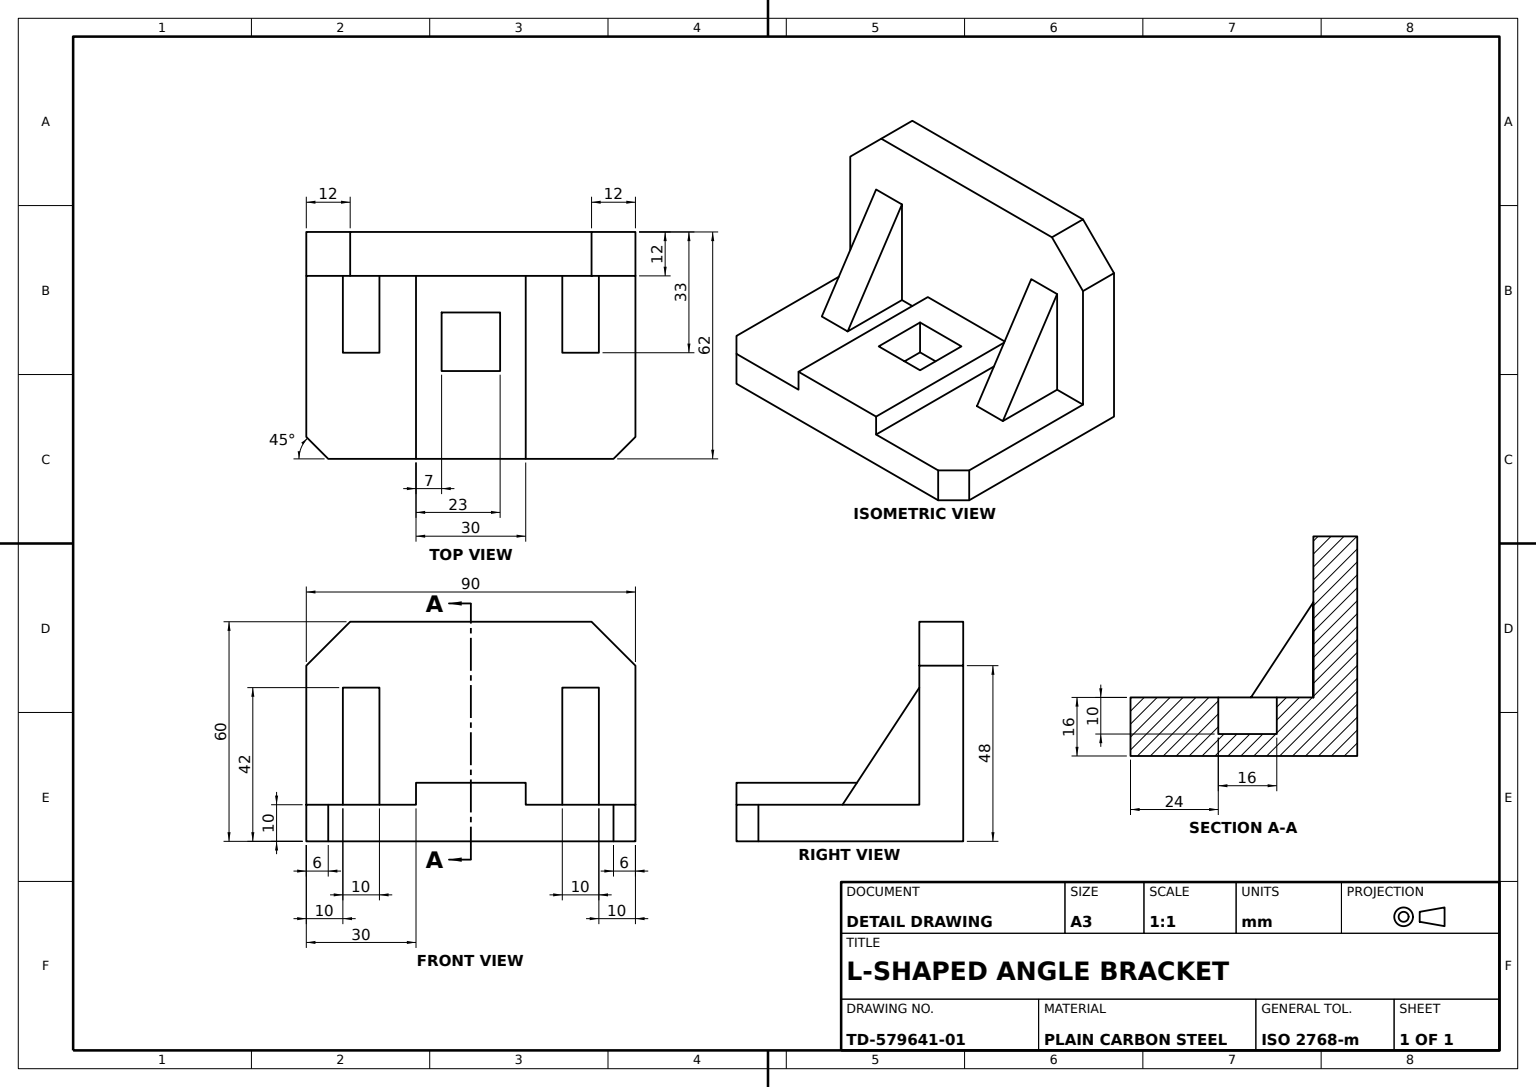
from build123d import *

# Parameters (mm, degrees)
BRACKET_BODY_DEPTH          = 12
CHAMFERED_PLATE_78X44_DEPTH = 10
CENTRE_PAD_SKETCH_W         = 30
CENTRE_PAD_SKETCH_H         = 50
CENTRE_PAD_30X30_DEPTH      = 6
PAD_POCKET_SKETCH_W         = 16
PAD_POCKET_SKETCH_H         = 16
PAD_POCKET_10X7_DEPTH       = 10
GUSSET_RIB_1_DEPTH          = 20
GUSSET_RIB_1_TRIM_DEPTH     = 10
GUSSET_RIB_2_DEPTH          = 20
GUSSET_RIB_2_TRIM_DEPTH     = 10


with BuildPart() as part:
    # Bracket Profile Sketch → Bracket Body (new body)
    with BuildSketch(Plane.XY):
        Polygon((3.579710145, 48), (3.579710145, 0), (93.579710145, 0), (93.579710145, 48), (81.579710145, 60), (15.579710145, 60), align=None)
    extrude(amount=BRACKET_BODY_DEPTH)

    # Chamfered Plate Sketch → Chamfered Plate 78x44 (add)
    with BuildSketch(Plane.XZ):
        Polygon((3.579710145, 12), (3.579710145, 56), (9.579710145, 62), (87.579710145, 62), (93.579710145, 56), (93.579710145, 12), align=None)
    extrude(amount=-CHAMFERED_PLATE_78X44_DEPTH)

    # Centre Pad Sketch → Centre Pad 30x30 (add)
    with BuildSketch(Plane(origin=(0, 10, 0), x_dir=(1, 0, 0), z_dir=(0, 1, 0))):
        with Locations((48.579710145, -37)):
            Rectangle(CENTRE_PAD_SKETCH_W, CENTRE_PAD_SKETCH_H)
    extrude(amount=CENTRE_PAD_30X30_DEPTH)

    # Pad Pocket Sketch → Pad Pocket 10x7 (cut)
    with BuildSketch(Plane(origin=(0, 16, 0), x_dir=(1, 0, 0), z_dir=(0, 1, 0))):
        with Locations((48.579710145, -30)):
            Rectangle(PAD_POCKET_SKETCH_W, PAD_POCKET_SKETCH_H)
    extrude(amount=-PAD_POCKET_10X7_DEPTH, mode=Mode.SUBTRACT)

    # Rib 1 Sketch → Gusset Rib 1 (add)
    with BuildSketch(Plane.ZY.offset(-3.579710145)):
        Polygon((12, 10), (12, 42), (33, 10), align=None)
    extrude(amount=-GUSSET_RIB_1_DEPTH)

    # Rib 1 Trim Sketch → Gusset Rib 1 Trim (cut)
    with BuildSketch(Plane.ZY.offset(-3.579710145)):
        Polygon((12, 42), (12, 10), (33, 10), align=None)
    extrude(amount=-GUSSET_RIB_1_TRIM_DEPTH, mode=Mode.SUBTRACT)

    # Rib 2 Sketch → Gusset Rib 2 (add)
    with BuildSketch(Plane(origin=(93.579710145, 0, 0), x_dir=(0, 0, -1), z_dir=(1, 0, 0))):
        Polygon((-12, 10), (-12, 42), (-33, 10), align=None)
    extrude(amount=-GUSSET_RIB_2_DEPTH)

    # Rib 2 Trim Sketch → Gusset Rib 2 Trim (cut)
    with BuildSketch(Plane(origin=(93.579710145, 0, 0), x_dir=(0, 0, -1), z_dir=(1, 0, 0))):
        Polygon((-12, 42), (-12, 10), (-33, 10), align=None)
    extrude(amount=-GUSSET_RIB_2_TRIM_DEPTH, mode=Mode.SUBTRACT)


solid = part.part
